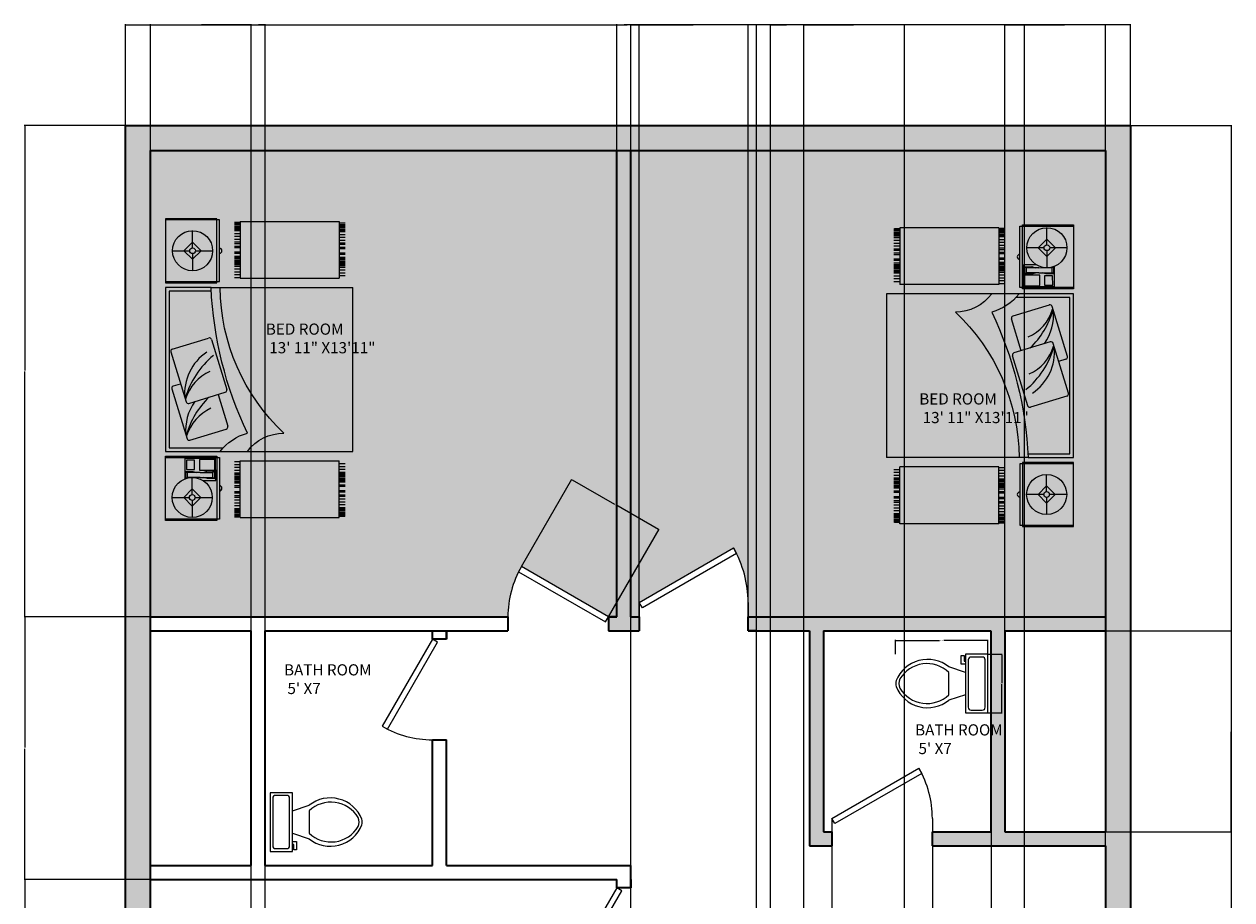
# Model space of a CAD drawing. Units: inches. Extents: x -29 to 404, y -32 to 761.
# Tile 5 of 5: x -29 to 404, y 447 to 761. Entities that reach past the tile are written whole.
import ezdxf

# ---------------------------------------------------------------- set-up
doc = ezdxf.new("R2010")
doc.units = ezdxf.units.IN
doc.header["$MEASUREMENT"] = 0
for name, color, linetype, lineweight in [('A-ANNO-DIMS', 2, 'Continuous', 18), ('A-AREA-IDEN', 7, 'Continuous', 18), ('A-FLOR-FIXT', 9, 'Continuous', 18), ('A-FURN', 8, 'Continuous', 18), ('A-WALL', 7, 'Continuous', 35), ('doors', 40, 'Continuous', 20)]:
    doc.layers.add(name, color=color, linetype=linetype, lineweight=lineweight)
doc.layers.add('A-WALL-PATT', color=251, linetype='Continuous', lineweight=13, true_color=0x636466)
doc.styles.get("Standard").update_dxf_attribs({"font": 'arial.ttf'})
doc.dimstyles.get("Standard").update_dxf_attribs({"dimtxt": 0.18, "dimasz": 0.18, "dimexe": 0.18, "dimexo": 0.0625, "dimgap": 0.09, "dimtad": 0, "dimtih": 1, "dimtoh": 1, "dimdec": 4, "dimzin": 0, "dimdsep": 46, "dimtxsty": 'Standard', "dimcen": 0.09, "dimadec": 0, "dimazin": 0, "dimtfac": 1, "dimtdec": 4, "dimtofl": 0, "dimtmove": 0, "dimatfit": 3, "dimfxl": 1, "dimtolj": 1, "dimtzin": 0, "dimarcsym": 0})

# ---------------------------------------------------------------- blocks, each defined once
blk = doc.blocks.new('3')
for p, q in [((185.866, 224.677), (185.866, 225.236)), ((185.866, 225.236), (186.566, 225.236)), ((185.88, 224.649), (185.88, 225.236)), ((186.552, 225.236), (186.552, 224.649)), ((186.566, 225.236), (186.566, 224.677)), ((186.62, 225.236), (186.62, 224.64)), ((188.409, 225.236), (186.62, 225.236)), ((187.706, 225.179), (187.161, 225.012)), ((188.409, 224.739), (188.409, 225.236)), ((188.463, 225.236), (188.463, 224.677)), ((189.162, 225.236), (188.463, 225.236)), ((188.477, 225.236), (188.477, 224.649)), ((189.148, 224.649), (189.148, 225.236)), ((189.162, 224.677), (189.162, 225.236)), ((186.022, 224.945), (186.116, 225.039)), ((186.116, 225.164), (186.116, 224.976)), ((186.116, 225.039), (186.21, 224.945)), ((187.303, 225.168), (186.758, 225.001)), ((187.334, 225.152), (187.359, 225.073)), ((187.737, 225.163), (187.858, 224.766)), ((188.812, 225.162), (188.812, 224.974)), ((186.084, 224.945), (185.896, 224.945)), ((186.116, 224.851), (186.022, 224.945)), ((186.21, 224.945), (186.116, 224.851)), ((186.116, 224.914), (186.116, 224.726)), ((186.147, 224.945), (186.335, 224.945)), ((186.54, 225.027), (186.319, 225.027)), ((186.321, 225.017), (186.401, 225.017)), ((186.333, 224.997), (186.321, 225.017)), ((186.334, 224.858), (186.333, 224.997)), ((186.333, 224.997), (186.389, 224.997)), ((186.401, 225.017), (186.389, 224.997)), ((186.39, 224.858), (186.389, 224.997)), ((186.401, 224.938), (186.389, 224.898)), ((186.401, 225.017), (186.401, 224.938)), ((186.541, 224.69), (186.54, 225.027)), ((186.742, 224.97), (186.863, 224.573)), ((187.144, 224.981), (187.266, 224.584)), ((188.781, 224.942), (188.593, 224.942)), ((188.812, 225.036), (188.718, 224.942)), ((188.718, 224.942), (188.812, 224.848)), ((188.907, 224.942), (188.812, 225.036)), ((188.812, 224.848), (188.907, 224.942)), ((188.812, 224.911), (188.812, 224.723)), ((188.844, 224.942), (189.032, 224.942)), ((186.302, 224.83), (186.303, 224.689)), ((186.322, 224.779), (186.334, 224.818)), ((186.323, 224.699), (186.322, 224.779)), ((186.331, 224.905), (186.334, 224.898)), ((186.334, 224.858), (186.334, 224.719)), ((186.39, 224.858), (186.39, 224.719)), ((186.402, 224.779), (186.39, 224.819)), ((186.402, 224.7), (186.402, 224.779)), ((186.566, 224.677), (185.866, 224.677)), ((186.552, 224.649), (185.88, 224.649)), ((186.303, 224.689), (186.541, 224.69)), ((186.334, 224.719), (186.323, 224.699)), ((186.323, 224.699), (186.402, 224.7)), ((186.334, 224.719), (186.39, 224.719)), ((186.402, 224.7), (186.39, 224.719)), ((187.242, 224.663), (186.894, 224.557)), ((187.842, 224.735), (187.297, 224.568)), ((188.409, 224.739), (188.409, 223.191)), ((188.463, 224.677), (189.162, 224.677)), ((188.477, 224.649), (189.148, 224.649)), ((186.62, 224.64), (186.62, 223.191)), ((185.897, 224.42, -0.909), (185.897, 223.338, -0.909)), ((185.897, 224.42, -0.909), (186.517, 224.42, -0.909)), ((185.904, 224.485, -0.909), (185.904, 224.42, -0.909)), ((185.92, 224.485, -0.909), (185.92, 224.42, -0.909)), ((185.92, 224.485, -0.909), (185.92, 224.42, -0.909)), ((185.935, 224.485, -0.909), (185.935, 224.42, -0.909)), ((185.951, 224.485, -0.909), (185.951, 224.42, -0.909)), ((185.966, 224.485, -0.909), (185.966, 224.42, -0.909)), ((185.982, 224.485, -0.909), (185.982, 224.42, -0.909)), ((185.997, 224.485, -0.909), (185.997, 224.42, -0.909)), ((186.028, 224.485, -0.909), (186.028, 224.42, -0.909)), ((186.059, 224.485, -0.909), (186.059, 224.42, -0.909)), ((186.09, 224.485, -0.909), (186.09, 224.42, -0.909)), ((186.09, 224.485, -0.909), (186.09, 224.42, -0.909)), ((186.121, 224.485, -0.909), (186.121, 224.42, -0.909)), ((186.137, 224.485, -0.909), (186.137, 224.42, -0.909)), ((186.168, 224.485, -0.909), (186.168, 224.42, -0.909)), ((186.183, 224.485, -0.909), (186.183, 224.42, -0.909)), ((186.23, 224.485, -0.909), (186.23, 224.42, -0.909)), ((186.245, 224.485, -0.909), (186.245, 224.42, -0.909)), ((186.276, 224.485, -0.909), (186.276, 224.42, -0.909)), ((186.292, 224.485, -0.909), (186.292, 224.42, -0.909)), ((186.307, 224.485, -0.909), (186.307, 224.42, -0.909)), ((186.323, 224.485, -0.909), (186.323, 224.42, -0.909)), ((186.338, 224.485, -0.909), (186.338, 224.42, -0.909)), ((186.354, 224.485, -0.909), (186.354, 224.42, -0.909)), ((186.369, 224.485, -0.909), (186.369, 224.42, -0.909)), ((186.385, 224.485, -0.909), (186.385, 224.42, -0.909)), ((186.416, 224.485, -0.909), (186.416, 224.42, -0.909)), ((186.447, 224.485, -0.909), (186.447, 224.42, -0.909)), ((186.478, 224.485, -0.909), (186.478, 224.42, -0.909)), ((186.509, 224.485, -0.909), (186.509, 224.42, -0.909)), ((186.517, 224.42, -0.909), (186.517, 223.338, -0.909)), ((189.131, 224.42, -0.909), (188.511, 224.42, -0.909)), ((188.511, 224.42, -0.909), (188.511, 223.338, -0.909)), ((188.52, 224.485, -0.909), (188.52, 224.42, -0.909)), ((188.551, 224.485, -0.909), (188.551, 224.42, -0.909)), ((188.582, 224.485, -0.909), (188.582, 224.42, -0.909)), ((188.613, 224.485, -0.909), (188.613, 224.42, -0.909)), ((188.644, 224.485, -0.909), (188.644, 224.42, -0.909)), ((188.66, 224.485, -0.909), (188.66, 224.42, -0.909)), ((188.675, 224.485, -0.909), (188.675, 224.42, -0.909)), ((188.691, 224.485, -0.909), (188.691, 224.42, -0.909)), ((188.706, 224.485, -0.909), (188.706, 224.42, -0.909)), ((188.722, 224.485, -0.909), (188.722, 224.42, -0.909)), ((188.737, 224.485, -0.909), (188.737, 224.42, -0.909)), ((188.753, 224.485, -0.909), (188.753, 224.42, -0.909)), ((188.784, 224.485, -0.909), (188.784, 224.42, -0.909)), ((188.799, 224.485, -0.909), (188.799, 224.42, -0.909)), ((188.846, 224.485, -0.909), (188.846, 224.42, -0.909)), ((188.861, 224.485, -0.909), (188.861, 224.42, -0.909)), ((188.892, 224.485, -0.909), (188.892, 224.42, -0.909)), ((188.908, 224.485, -0.909), (188.908, 224.42, -0.909)), ((188.939, 224.485, -0.909), (188.939, 224.42, -0.909)), ((188.939, 224.485, -0.909), (188.939, 224.42, -0.909)), ((188.97, 224.485, -0.909), (188.97, 224.42, -0.909)), ((189.001, 224.485, -0.909), (189.001, 224.42, -0.909)), ((189.032, 224.485, -0.909), (189.032, 224.42, -0.909)), ((189.047, 224.485, -0.909), (189.047, 224.42, -0.909)), ((189.063, 224.485, -0.909), (189.063, 224.42, -0.909)), ((189.078, 224.485, -0.909), (189.078, 224.42, -0.909)), ((189.094, 224.485, -0.909), (189.094, 224.42, -0.909)), ((189.109, 224.485, -0.909), (189.109, 224.42, -0.909)), ((189.109, 224.485, -0.909), (189.109, 224.42, -0.909)), ((189.125, 224.485, -0.909), (189.125, 224.42, -0.909)), ((189.131, 224.42, -0.909), (189.131, 223.338, -0.909)), ((185.897, 223.338, -0.909), (186.517, 223.338, -0.909)), ((185.911, 223.338, -0.909), (185.911, 223.279, -0.909)), ((185.911, 223.338, -0.909), (185.911, 223.279, -0.909)), ((185.911, 223.338, -0.909), (185.911, 223.279, -0.909)), ((185.914, 223.338, -0.909), (185.914, 223.273, -0.909)), ((185.929, 223.338, -0.909), (185.929, 223.273, -0.909)), ((185.929, 223.338, -0.909), (185.929, 223.273, -0.909)), ((185.945, 223.338, -0.909), (185.945, 223.273, -0.909)), ((185.96, 223.338, -0.909), (185.96, 223.273, -0.909)), ((185.976, 223.338, -0.909), (185.976, 223.273, -0.909)), ((185.991, 223.338, -0.909), (185.991, 223.273, -0.909)), ((186.007, 223.338, -0.909), (186.007, 223.273, -0.909)), ((186.038, 223.338, -0.909), (186.038, 223.273, -0.909)), ((186.069, 223.338, -0.909), (186.069, 223.273, -0.909)), ((186.1, 223.338, -0.909), (186.1, 223.273, -0.909)), ((186.1, 223.338, -0.909), (186.1, 223.273, -0.909)), ((186.131, 223.338, -0.909), (186.131, 223.273, -0.909)), ((186.146, 223.338, -0.909), (186.146, 223.273, -0.909)), ((186.177, 223.338, -0.909), (186.177, 223.273, -0.909)), ((186.193, 223.338, -0.909), (186.193, 223.273, -0.909)), ((186.239, 223.338, -0.909), (186.239, 223.273, -0.909)), ((186.255, 223.338, -0.909), (186.255, 223.273, -0.909)), ((186.286, 223.338, -0.909), (186.286, 223.273, -0.909)), ((186.301, 223.338, -0.909), (186.301, 223.273, -0.909)), ((186.317, 223.338, -0.909), (186.317, 223.273, -0.909)), ((186.332, 223.338, -0.909), (186.332, 223.273, -0.909)), ((186.348, 223.338, -0.909), (186.348, 223.273, -0.909)), ((186.363, 223.338, -0.909), (186.363, 223.273, -0.909)), ((186.379, 223.338, -0.909), (186.379, 223.273, -0.909)), ((186.394, 223.338, -0.909), (186.394, 223.273, -0.909)), ((186.425, 223.338, -0.909), (186.425, 223.273, -0.909)), ((186.456, 223.338, -0.909), (186.456, 223.273, -0.909)), ((186.487, 223.338, -0.909), (186.487, 223.273, -0.909)), ((189.131, 223.338, -0.909), (188.511, 223.338, -0.909)), ((188.541, 223.338, -0.909), (188.541, 223.273, -0.909)), ((188.572, 223.338, -0.909), (188.572, 223.273, -0.909)), ((188.603, 223.338, -0.909), (188.603, 223.273, -0.909)), ((188.634, 223.338, -0.909), (188.634, 223.273, -0.909)), ((188.65, 223.338, -0.909), (188.65, 223.273, -0.909)), ((188.665, 223.338, -0.909), (188.665, 223.273, -0.909)), ((188.681, 223.338, -0.909), (188.681, 223.273, -0.909)), ((188.696, 223.338, -0.909), (188.696, 223.273, -0.909)), ((188.712, 223.338, -0.909), (188.712, 223.273, -0.909)), ((188.727, 223.338, -0.909), (188.727, 223.273, -0.909)), ((188.743, 223.338, -0.909), (188.743, 223.273, -0.909)), ((188.774, 223.338, -0.909), (188.774, 223.273, -0.909)), ((188.789, 223.338, -0.909), (188.789, 223.273, -0.909)), ((188.836, 223.338, -0.909), (188.836, 223.273, -0.909)), ((188.851, 223.338, -0.909), (188.851, 223.273, -0.909)), ((188.882, 223.338, -0.909), (188.882, 223.273, -0.909)), ((188.898, 223.338, -0.909), (188.898, 223.273, -0.909)), ((188.929, 223.338, -0.909), (188.929, 223.273, -0.909)), ((188.929, 223.338, -0.909), (188.929, 223.273, -0.909)), ((188.96, 223.338, -0.909), (188.96, 223.273, -0.909)), ((188.991, 223.338, -0.909), (188.991, 223.273, -0.909)), ((189.022, 223.338, -0.909), (189.022, 223.273, -0.909)), ((189.037, 223.338, -0.909), (189.037, 223.273, -0.909)), ((189.053, 223.338, -0.909), (189.053, 223.273, -0.909)), ((189.068, 223.338, -0.909), (189.068, 223.273, -0.909)), ((189.084, 223.338, -0.909), (189.084, 223.273, -0.909)), ((189.099, 223.338, -0.909), (189.099, 223.273, -0.909)), ((189.099, 223.338, -0.909), (189.099, 223.273, -0.909)), ((189.115, 223.338, -0.909), (189.115, 223.273, -0.909)), ((189.117, 223.338, -0.909), (189.117, 223.279, -0.909)), ((189.117, 223.338, -0.909), (189.117, 223.279, -0.909)), ((189.117, 223.338, -0.909), (189.117, 223.279, -0.909)), ((186.62, 223.191), (188.409, 223.191))]:
    blk.add_line(p, q)
blk.add_lwpolyline([(188.369, 224.737), (188.369, 225.197), (186.66, 225.197), (186.66, 224.606)])
for points in [[(186.422, 225.007), (186.422, 224.92), (186.525, 224.92), (186.525, 225.008)], [(186.415, 224.866), (186.416, 224.7), (186.531, 224.7), (186.53, 224.867)]]:
    blk.add_lwpolyline(points, close=True)
for points in [[(186.62, 224.64, -0.162278), (186.819, 224.342, -0.100664), (188.409, 224.739, -0.100664)], [(186.62, 224.342, -0.236068), (186.819, 223.944, -0.205258), (188.409, 224.64, -0.205258)]]:
    blk.add_lwpolyline(points, format="xyb")
for centre, radius in [((186.116, 224.945), 0.219), ((188.812, 224.942), 0.219), ((186.116, 224.945), 0.0313), ((188.812, 224.942), 0.0313)]:
    blk.add_circle(centre, radius)
for centre, radius, start, end in [((187.713, 225.156), 0.0248, 17.0142, 107.0142), ((187.311, 225.145), 0.0248, 17.0142, 107.0142), ((186.765, 224.978), 0.0248, 107.0142, 197.0142), ((186.647, 224.541), 0.487, 24.2209, 73.0691), ((186.848, 224.471), 0.547, 54.6851, 95.1605), ((186.536, 224.105), 0.943, 44.2727, 73.7189), ((187.168, 224.989), 0.0248, 107.0142, 197.0142), ((187.05, 224.552), 0.487, 24.2209, 73.0691), ((187.25, 224.482), 0.547, 33.7801, 95.1605), ((186.938, 224.116), 0.943, 39.4023, 73.7189), ((186.216, 224.649), 0.028, 180, 0), ((187.835, 224.758), 0.0248, 287.0142, 17.0142), ((188.812, 224.649), 0.028, 180, 0), ((186.887, 224.581), 0.0248, 197.0142, 287.0142), ((187.289, 224.592), 0.0248, 197.0142, 287.0142)]:
    blk.add_arc(centre, radius, start, end)
blk = doc.blocks.new('Toilet - top')
for p, q in [((9.5, -6), (9.5, -2)), ((-10, -8.5), (-8, -8.5)), ((-10, -9.5), (-10, -8.5)), ((-8, -8.5), (-8, -8)), ((-7, -8), (-7, -9.5)), ((-4, -8), (-6, -14)), ((4, -8), (6, -14)), ((-7, -9.5), (-10, -9.5)), ((4, -14), (-4, -14))]:
    blk.add_line(p, q)
blk.add_lwpolyline([(10.5, -8), (10.5, 0), (-10.5, 0), (-10.5, -8)], close=True)
for points in [[(-9.5, -2), (-9.5, -6)], [(8.5, -1), (-8.5, -1)], [(-8.5, -7), (8.5, -7)]]:
    blk.add_lwpolyline(points)
for centre, radius, start, end in [((-8.62, -1.88), 0.884, 81.8699, 188.1301), ((8.62, -1.88), 0.884, 351.8699, 98.1301), ((-8.62, -6.12), 0.884, 171.8699, 278.1301), ((8.62, -6.12), 0.884, 261.8699, 8.1301), ((3.52, -21.58), 12.17, 141.4691, 247.9714), ((4.2, -21.82), 11.33, 136.3677, 238.9468), ((-3.52, -21.58), 12.17, 292.0284, 38.5307), ((-4.2, -21.82), 11.33, 301.053, 43.6321), ((0, -27.88), 4, 245.7318, 294.2682), ((0, -29), 4, 254.8605, 285.1395)]:
    blk.add_arc(centre, radius, start, end)
blk = doc.blocks.new('*U7')
for p, q in [((0, 0), (0, 100)), ((750, 0), (750, 100))]:
    blk.add_line(p, q)
blk.add_lwpolyline([(0, 0), (649.5, -375), (671.4, -337.1), (21.9, 37.9)], close=True)
blk.add_arc((0, 0), 750, 330, 0)
blk = doc.blocks.new('*U6')
for p, q in [((0, 0), (0, -100)), ((750, 0), (750, -100))]:
    blk.add_line(p, q)
blk.add_lwpolyline([(0, 0), (649.5, 375), (671.4, 337.1), (21.9, -37.9)], close=True)
blk.add_arc((0, 0), 750, 0, 30)
blk = doc.blocks.new('*D15')
at = {"layer": 'A-ANNO-DIMS', "color": 0, "lineweight": -2, "transparency": 16777216}
for p, q in [((283.5, 535.13), (283.5, 540.2)), ((283.68, 540.02), (299.25, 540.02)), ((316.37, 540.02), (300.8, 540.02)), ((316.55, 535.13), (316.55, 540.2))]:
    blk.add_line(p, q, dxfattribs=at)
at = {"layer": 'A-ANNO-DIMS', "color": 0, "transparency": 16777216}
for points in [[(283.68, 540.05), (283.68, 539.99), (283.5, 540.02)], [(316.37, 540.05), (316.37, 539.99), (316.55, 540.02)]]:
    blk.add_solid(points, dxfattribs=at)
at = {"layer": 'Defpoints', "color": 0, "transparency": 16777216}
for p in [(316.55, 540.02), (283.5, 535.07), (316.55, 535.07)]:
    blk.add_point(p, dxfattribs=at)
at = {"layer": 'A-ANNO-DIMS', "color": 0, "transparency": 16777216, "insert": (300.03, 540.02), "char_height": 0.18, "attachment_point": 5}
blk.add_mtext('\\A1;WC 33 TYP.', dxfattribs=at)
blk = doc.blocks.new('*D16')
at = {"layer": 'A-ANNO-DIMS', "color": 0, "lineweight": -2, "transparency": 16777216}
for p, q in [((316.61, 535.07), (321.69, 535.07)), ((321.51, 534.89), (321.51, 524.75)), ((321.51, 514.25), (321.51, 524.39)), ((316.61, 514.07), (321.69, 514.07))]:
    blk.add_line(p, q, dxfattribs=at)
at = {"layer": 'A-ANNO-DIMS', "color": 0, "transparency": 16777216}
for points in [[(321.48, 534.89), (321.54, 534.89), (321.51, 535.07)], [(321.48, 514.25), (321.54, 514.25), (321.51, 514.07)]]:
    blk.add_solid(points, dxfattribs=at)
at = {"layer": 'Defpoints', "color": 0, "transparency": 16777216}
for p in [(316.55, 535.07), (316.55, 514.07), (321.51, 514.07)]:
    blk.add_point(p, dxfattribs=at)
at = {"layer": 'A-ANNO-DIMS', "color": 0, "transparency": 16777216, "insert": (321.51, 524.57), "char_height": 0.18, "attachment_point": 5}
blk.add_mtext('\\A1;21 TYP.', dxfattribs=at)
blk = doc.blocks.new('*D31')
at = {"layer": 'A-ANNO-DIMS', "color": 0, "lineweight": -2, "transparency": 16777216}
for p, q in [((7.68, 724.5), (7.68, 760.66)), ((7.86, 760.48), (187.39, 760.48)), ((367.5, 760.48), (187.97, 760.48)), ((367.68, 724.5), (367.68, 760.66))]:
    blk.add_line(p, q, dxfattribs=at)
at = {"layer": 'A-ANNO-DIMS', "color": 0, "transparency": 16777216}
for points in [[(7.86, 760.51), (7.86, 760.45), (7.68, 760.48)], [(367.5, 760.51), (367.5, 760.45), (367.68, 760.48)]]:
    blk.add_solid(points, dxfattribs=at)
at = {"layer": 'Defpoints', "color": 0, "transparency": 16777216}
for p in [(367.68, 760.48), (7.68, 724.43), (367.68, 724.43)]:
    blk.add_point(p, dxfattribs=at)
at = {"layer": 'A-ANNO-DIMS', "color": 0, "transparency": 16777216, "insert": (187.68, 760.48), "char_height": 0.18, "attachment_point": 5}
blk.add_mtext('\\A1;360', dxfattribs=at)
blk = doc.blocks.new('*D32')
at = {"layer": 'A-ANNO-DIMS', "color": 0, "lineweight": -2, "transparency": 16777216}
for p, q in [((367.74, 724.43), (403.91, 724.43)), ((403.73, 724.25), (403.73, 364.62)), ((403.73, 4.61), (403.73, 364.25)), ((367.74, 4.43), (403.91, 4.43))]:
    blk.add_line(p, q, dxfattribs=at)
at = {"layer": 'A-ANNO-DIMS', "color": 0, "transparency": 16777216}
for points in [[(403.7, 724.25), (403.76, 724.25), (403.73, 724.43)], [(403.7, 4.61), (403.76, 4.61), (403.73, 4.43)]]:
    blk.add_solid(points, dxfattribs=at)
at = {"layer": 'Defpoints', "color": 0, "transparency": 16777216}
for p in [(367.68, 724.43), (403.73, 724.43), (367.68, 4.43)]:
    blk.add_point(p, dxfattribs=at)
at = {"layer": 'A-ANNO-DIMS', "color": 0, "transparency": 16777216, "insert": (403.73, 364.43), "char_height": 0.18, "attachment_point": 5}
blk.add_mtext('\\A1;720', dxfattribs=at)
blk = doc.blocks.new('*D35')
at = {"layer": 'A-ANNO-DIMS', "color": 0, "lineweight": -2, "transparency": 16777216}
for p, q in [((16.62, 454.43), (-28.55, 454.43)), ((-28.37, 454.25), (-28.37, 371.12)), ((-28.37, 287.61), (-28.37, 370.75)), ((16.62, 287.43), (-28.55, 287.43))]:
    blk.add_line(p, q, dxfattribs=at)
at = {"layer": 'A-ANNO-DIMS', "color": 0, "transparency": 16777216}
for points in [[(-28.4, 454.25), (-28.34, 454.25), (-28.37, 454.43)], [(-28.4, 287.61), (-28.34, 287.61), (-28.37, 287.43)]]:
    blk.add_solid(points, dxfattribs=at)
at = {"layer": 'Defpoints', "color": 0, "transparency": 16777216}
for p in [(-28.37, 454.43), (16.68, 454.43), (16.68, 287.43)]:
    blk.add_point(p, dxfattribs=at)
at = {"layer": 'A-ANNO-DIMS', "color": 0, "transparency": 16777216, "insert": (-28.37, 370.93), "char_height": 0.18, "attachment_point": 5}
blk.add_mtext('\\A1;167', dxfattribs=at)
blk = doc.blocks.new('*D36')
at = {"layer": 'A-ANNO-DIMS', "color": 0, "lineweight": -2, "transparency": 16777216}
for p, q in [((16.62, 548.43), (-28.55, 548.43)), ((-28.37, 548.25), (-28.37, 501.62)), ((-28.37, 454.61), (-28.37, 501.25)), ((16.62, 454.43), (-28.55, 454.43))]:
    blk.add_line(p, q, dxfattribs=at)
at = {"layer": 'A-ANNO-DIMS', "color": 0, "transparency": 16777216}
for points in [[(-28.4, 548.25), (-28.34, 548.25), (-28.37, 548.43)], [(-28.4, 454.61), (-28.34, 454.61), (-28.37, 454.43)]]:
    blk.add_solid(points, dxfattribs=at)
at = {"layer": 'Defpoints', "color": 0, "transparency": 16777216}
for p in [(-28.37, 548.43), (16.68, 548.43), (16.68, 454.43)]:
    blk.add_point(p, dxfattribs=at)
at = {"layer": 'A-ANNO-DIMS', "color": 0, "transparency": 16777216, "insert": (-28.37, 501.43), "char_height": 0.18, "attachment_point": 5}
blk.add_mtext('\\A1;94', dxfattribs=at)
blk = doc.blocks.new('*D37')
at = {"layer": 'A-ANNO-DIMS', "color": 0, "lineweight": -2, "transparency": 16777216}
for p, q in [((7.62, 724.43), (-28.55, 724.43)), ((-28.37, 724.25), (-28.37, 636.62)), ((-28.37, 548.61), (-28.37, 636.25)), ((16.62, 548.43), (-28.55, 548.43))]:
    blk.add_line(p, q, dxfattribs=at)
at = {"layer": 'A-ANNO-DIMS', "color": 0, "transparency": 16777216}
for points in [[(-28.4, 724.25), (-28.34, 724.25), (-28.37, 724.43)], [(-28.4, 548.61), (-28.34, 548.61), (-28.37, 548.43)]]:
    blk.add_solid(points, dxfattribs=at)
at = {"layer": 'Defpoints', "color": 0, "transparency": 16777216}
for p in [(-28.37, 724.43), (7.68, 724.43), (16.68, 548.43)]:
    blk.add_point(p, dxfattribs=at)
at = {"layer": 'A-ANNO-DIMS', "color": 0, "transparency": 16777216, "insert": (-28.37, 636.43), "char_height": 0.18, "attachment_point": 5}
blk.add_mtext('\\A1;176', dxfattribs=at)
blk = doc.blocks.new('*D41')
at = {"layer": 'A-ANNO-DIMS', "color": 0, "lineweight": -2, "transparency": 16777216}
for p, q in [((250.68, 193.5), (250.68, 760.66)), ((250.86, 760.48), (268.46, 760.48)), ((286.5, 760.48), (268.9, 760.48)), ((286.68, 193.5), (286.68, 760.66))]:
    blk.add_line(p, q, dxfattribs=at)
at = {"layer": 'A-ANNO-DIMS', "color": 0, "transparency": 16777216}
for points in [[(250.86, 760.51), (250.86, 760.45), (250.68, 760.48)], [(286.5, 760.51), (286.5, 760.45), (286.68, 760.48)]]:
    blk.add_solid(points, dxfattribs=at)
at = {"layer": 'Defpoints', "color": 0, "transparency": 16777216}
for p in [(286.68, 760.48), (250.68, 193.43), (286.68, 193.43)]:
    blk.add_point(p, dxfattribs=at)
at = {"layer": 'A-ANNO-DIMS', "color": 0, "transparency": 16777216, "insert": (268.68, 760.48), "char_height": 0.18, "attachment_point": 5}
blk.add_mtext('\\A1;36', dxfattribs=at)
blk = doc.blocks.new('*D42')
at = {"layer": 'A-ANNO-DIMS', "color": 0, "lineweight": -2, "transparency": 16777216}
for p, q in [((238.68, 193.5), (238.68, 760.66)), ((238.86, 760.48), (244.47, 760.48)), ((250.5, 760.48), (244.89, 760.48)), ((250.68, 193.5), (250.68, 760.66))]:
    blk.add_line(p, q, dxfattribs=at)
at = {"layer": 'A-ANNO-DIMS', "color": 0, "transparency": 16777216}
for points in [[(238.86, 760.51), (238.86, 760.45), (238.68, 760.48)], [(250.5, 760.51), (250.5, 760.45), (250.68, 760.48)]]:
    blk.add_solid(points, dxfattribs=at)
at = {"layer": 'Defpoints', "color": 0, "transparency": 16777216}
for p in [(250.68, 760.48), (238.68, 193.43), (250.68, 193.43)]:
    blk.add_point(p, dxfattribs=at)
at = {"layer": 'A-ANNO-DIMS', "color": 0, "transparency": 16777216, "insert": (244.68, 760.48), "char_height": 0.18, "attachment_point": 5}
blk.add_mtext('\\A1;12', dxfattribs=at)
blk = doc.blocks.new('*D44')
at = {"layer": 'A-ANNO-DIMS', "color": 0, "lineweight": -2, "transparency": 16777216}
for p, q in [((188.68, 92.5), (188.68, 760.66)), ((188.86, 760.48), (210.95, 760.48)), ((233.5, 760.48), (211.4, 760.48)), ((233.68, 92.5), (233.68, 760.66))]:
    blk.add_line(p, q, dxfattribs=at)
at = {"layer": 'A-ANNO-DIMS', "color": 0, "transparency": 16777216}
for points in [[(188.86, 760.51), (188.86, 760.45), (188.68, 760.48)], [(233.5, 760.51), (233.5, 760.45), (233.68, 760.48)]]:
    blk.add_solid(points, dxfattribs=at)
at = {"layer": 'Defpoints', "color": 0, "transparency": 16777216}
for p in [(233.68, 760.48), (188.68, 92.43), (233.68, 92.43)]:
    blk.add_point(p, dxfattribs=at)
at = {"layer": 'A-ANNO-DIMS', "color": 0, "transparency": 16777216, "insert": (211.18, 760.48), "char_height": 0.18, "attachment_point": 5}
blk.add_mtext('\\A1;45', dxfattribs=at)
blk = doc.blocks.new('*D45')
at = {"layer": 'A-ANNO-DIMS', "color": 0, "lineweight": -2, "transparency": 16777216}
for p, q in [((329.68, 126.5), (329.68, 760.66)), ((329.86, 760.48), (343.96, 760.48)), ((358.5, 760.48), (344.4, 760.48)), ((358.68, 97.5), (358.68, 760.66))]:
    blk.add_line(p, q, dxfattribs=at)
at = {"layer": 'A-ANNO-DIMS', "color": 0, "transparency": 16777216}
for points in [[(329.86, 760.51), (329.86, 760.45), (329.68, 760.48)], [(358.5, 760.51), (358.5, 760.45), (358.68, 760.48)]]:
    blk.add_solid(points, dxfattribs=at)
at = {"layer": 'Defpoints', "color": 0, "transparency": 16777216}
for p in [(358.68, 760.48), (329.68, 126.43), (358.68, 97.43)]:
    blk.add_point(p, dxfattribs=at)
at = {"layer": 'A-ANNO-DIMS', "color": 0, "transparency": 16777216, "insert": (344.18, 760.48), "char_height": 0.18, "attachment_point": 5}
blk.add_mtext('\\A1;29', dxfattribs=at)
blk = doc.blocks.new('*D48')
at = {"layer": 'A-ANNO-DIMS', "color": 0, "lineweight": -2, "transparency": 16777216}
for p, q in [((183.68, 715.5), (183.68, 760.66)), ((183.86, 760.48), (186.03, 760.48)), ((188.5, 760.48), (186.33, 760.48)), ((188.68, 715.5), (188.68, 760.66))]:
    blk.add_line(p, q, dxfattribs=at)
at = {"layer": 'A-ANNO-DIMS', "color": 0, "transparency": 16777216}
for points in [[(183.86, 760.51), (183.86, 760.45), (183.68, 760.48)], [(188.5, 760.51), (188.5, 760.45), (188.68, 760.48)]]:
    blk.add_solid(points, dxfattribs=at)
at = {"layer": 'Defpoints', "color": 0, "transparency": 16777216}
for p in [(188.68, 760.48), (183.68, 715.43), (188.68, 715.43)]:
    blk.add_point(p, dxfattribs=at)
at = {"layer": 'A-ANNO-DIMS', "color": 0, "transparency": 16777216, "insert": (186.18, 760.48), "char_height": 0.18, "attachment_point": 5}
blk.add_mtext('\\A1;5', dxfattribs=at)
blk = doc.blocks.new('*D50')
at = {"layer": 'A-ANNO-DIMS', "color": 0, "lineweight": -2, "transparency": 16777216}
for p, q in [((260.68, 466.37), (260.68, -31.8)), ((296.68, 466.37), (296.68, -31.8)), ((260.86, -31.62), (278.46, -31.62)), ((296.5, -31.62), (278.9, -31.62))]:
    blk.add_line(p, q, dxfattribs=at)
at = {"layer": 'A-ANNO-DIMS', "color": 0, "transparency": 16777216}
for points in [[(260.86, -31.59), (260.86, -31.65), (260.68, -31.62)], [(296.5, -31.59), (296.5, -31.65), (296.68, -31.62)]]:
    blk.add_solid(points, dxfattribs=at)
at = {"layer": 'Defpoints', "color": 0, "transparency": 16777216}
for p in [(260.68, 466.43), (296.68, 466.43), (296.68, -31.62)]:
    blk.add_point(p, dxfattribs=at)
at = {"layer": 'A-ANNO-DIMS', "color": 0, "transparency": 16777216, "insert": (278.68, -31.62), "char_height": 0.18, "attachment_point": 5}
blk.add_mtext('\\A1;36', dxfattribs=at)
blk = doc.blocks.new('*D51')
at = {"layer": 'A-ANNO-DIMS', "color": 0, "lineweight": -2, "transparency": 16777216}
for p, q in [((296.68, 471.37), (296.68, -31.8)), ((317.68, 471.37), (317.68, -31.8)), ((296.86, -31.62), (306.97, -31.62)), ((317.5, -31.62), (307.38, -31.62))]:
    blk.add_line(p, q, dxfattribs=at)
at = {"layer": 'A-ANNO-DIMS', "color": 0, "transparency": 16777216}
for points in [[(296.86, -31.59), (296.86, -31.65), (296.68, -31.62)], [(317.5, -31.59), (317.5, -31.65), (317.68, -31.62)]]:
    blk.add_solid(points, dxfattribs=at)
at = {"layer": 'Defpoints', "color": 0, "transparency": 16777216}
for p in [(296.68, 471.43), (317.68, 471.43), (317.68, -31.62)]:
    blk.add_point(p, dxfattribs=at)
at = {"layer": 'A-ANNO-DIMS', "color": 0, "transparency": 16777216, "insert": (307.18, -31.62), "char_height": 0.18, "attachment_point": 5}
blk.add_mtext('\\A1;21', dxfattribs=at)
blk = doc.blocks.new('*D52')
at = {"layer": 'A-ANNO-DIMS', "color": 0, "lineweight": -2, "transparency": 16777216}
for p, q in [((358.74, 543.43), (403.91, 543.43)), ((403.73, 543.25), (403.73, 507.61)), ((403.73, 471.61), (403.73, 507.25)), ((358.74, 471.43), (403.91, 471.43))]:
    blk.add_line(p, q, dxfattribs=at)
at = {"layer": 'A-ANNO-DIMS', "color": 0, "transparency": 16777216}
for points in [[(403.7, 543.25), (403.76, 543.25), (403.73, 543.43)], [(403.7, 471.61), (403.76, 471.61), (403.73, 471.43)]]:
    blk.add_solid(points, dxfattribs=at)
at = {"layer": 'Defpoints', "color": 0, "transparency": 16777216}
for p in [(358.68, 543.43), (403.73, 543.43), (358.68, 471.43)]:
    blk.add_point(p, dxfattribs=at)
at = {"layer": 'A-ANNO-DIMS', "color": 0, "transparency": 16777216, "insert": (403.73, 507.43), "char_height": 0.18, "attachment_point": 5}
blk.add_mtext('\\A1;72', dxfattribs=at)
blk = doc.blocks.new('*D53')
at = {"layer": 'A-ANNO-DIMS', "color": 0, "lineweight": -2, "transparency": 16777216}
for p, q in [((322.68, 543.5), (322.68, 760.66)), ((322.86, 760.48), (340.46, 760.48)), ((358.5, 760.48), (340.9, 760.48)), ((358.68, 543.5), (358.68, 760.66))]:
    blk.add_line(p, q, dxfattribs=at)
at = {"layer": 'A-ANNO-DIMS', "color": 0, "transparency": 16777216}
for points in [[(322.86, 760.51), (322.86, 760.45), (322.68, 760.48)], [(358.5, 760.51), (358.5, 760.45), (358.68, 760.48)]]:
    blk.add_solid(points, dxfattribs=at)
at = {"layer": 'Defpoints', "color": 0, "transparency": 16777216}
for p in [(358.68, 760.48), (322.68, 543.43), (358.68, 543.43)]:
    blk.add_point(p, dxfattribs=at)
at = {"layer": 'A-ANNO-DIMS', "color": 0, "transparency": 16777216, "insert": (340.68, 760.48), "char_height": 0.18, "attachment_point": 5}
blk.add_mtext('\\A1;36', dxfattribs=at)
blk = doc.blocks.new('*D56')
at = {"layer": 'A-ANNO-DIMS', "color": 0, "lineweight": -2, "transparency": 16777216}
for p, q in [((149.53, 566.49), (167.62, 597.81)), ((167.68, 597.56), (182.9, 588.78)), ((198.55, 579.74), (183.33, 588.53)), ((180.71, 548.49), (198.79, 579.81))]:
    blk.add_line(p, q, dxfattribs=at)
at = {"layer": 'A-ANNO-DIMS', "color": 0, "transparency": 16777216}
for points in [[(167.7, 597.59), (167.67, 597.54), (167.53, 597.65)], [(198.56, 579.77), (198.53, 579.72), (198.7, 579.65)]]:
    blk.add_solid(points, dxfattribs=at)
at = {"layer": 'Defpoints', "color": 0, "transparency": 16777216}
for p in [(198.7, 579.65), (149.5, 566.43), (180.68, 548.43)]:
    blk.add_point(p, dxfattribs=at)
at = {"layer": 'A-ANNO-DIMS', "color": 0, "transparency": 16777216, "insert": (183.11, 588.65), "char_height": 0.18, "attachment_point": 5}
blk.add_mtext('\\A1;36', dxfattribs=at)
blk = doc.blocks.new('*D57')
at = {"layer": 'A-ANNO-DIMS', "color": 0, "lineweight": -2, "transparency": 16777216}
for p, q in [((191.68, 543.5), (191.68, 760.66)), ((191.86, 760.48), (210.96, 760.48)), ((230.5, 760.48), (211.4, 760.48)), ((230.68, 543.5), (230.68, 760.66))]:
    blk.add_line(p, q, dxfattribs=at)
at = {"layer": 'A-ANNO-DIMS', "color": 0, "transparency": 16777216}
for points in [[(191.86, 760.51), (191.86, 760.45), (191.68, 760.48)], [(230.5, 760.51), (230.5, 760.45), (230.68, 760.48)]]:
    blk.add_solid(points, dxfattribs=at)
at = {"layer": 'Defpoints', "color": 0, "transparency": 16777216}
for p in [(230.68, 760.48), (191.68, 543.43), (230.68, 543.43)]:
    blk.add_point(p, dxfattribs=at)
at = {"layer": 'A-ANNO-DIMS', "color": 0, "transparency": 16777216, "insert": (211.18, 760.48), "char_height": 0.18, "attachment_point": 5}
blk.add_mtext('\\A1;39', dxfattribs=at)
blk = doc.blocks.new('*D59')
at = {"layer": 'A-ANNO-DIMS', "color": 0, "lineweight": -2, "transparency": 16777216}
for p, q in [((16.68, 198.5), (16.68, 760.66)), ((16.86, 760.48), (34.46, 760.48)), ((52.5, 760.48), (34.9, 760.48)), ((52.68, 198.5), (52.68, 760.66))]:
    blk.add_line(p, q, dxfattribs=at)
at = {"layer": 'A-ANNO-DIMS', "color": 0, "transparency": 16777216}
for points in [[(16.86, 760.51), (16.86, 760.45), (16.68, 760.48)], [(52.5, 760.51), (52.5, 760.45), (52.68, 760.48)]]:
    blk.add_solid(points, dxfattribs=at)
at = {"layer": 'Defpoints', "color": 0, "transparency": 16777216}
for p in [(52.68, 760.48), (16.68, 198.43), (52.68, 198.43)]:
    blk.add_point(p, dxfattribs=at)
at = {"layer": 'A-ANNO-DIMS', "color": 0, "transparency": 16777216, "insert": (34.68, 760.48), "char_height": 0.18, "attachment_point": 5}
blk.add_mtext('\\A1;36', dxfattribs=at)
blk = doc.blocks.new('*D60')
at = {"layer": 'A-ANNO-DIMS', "color": 0, "lineweight": -2, "transparency": 16777216}
for p, q in [((52.68, 198.5), (52.68, 760.66)), ((52.86, 760.48), (55.03, 760.48)), ((57.5, 760.48), (55.33, 760.48)), ((57.68, 198.5), (57.68, 760.66))]:
    blk.add_line(p, q, dxfattribs=at)
at = {"layer": 'A-ANNO-DIMS', "color": 0, "transparency": 16777216}
for points in [[(52.86, 760.51), (52.86, 760.45), (52.68, 760.48)], [(57.5, 760.51), (57.5, 760.45), (57.68, 760.48)]]:
    blk.add_solid(points, dxfattribs=at)
at = {"layer": 'Defpoints', "color": 0, "transparency": 16777216}
for p in [(57.68, 760.48), (52.68, 198.43), (57.68, 198.43)]:
    blk.add_point(p, dxfattribs=at)
at = {"layer": 'A-ANNO-DIMS', "color": 0, "transparency": 16777216, "insert": (55.18, 760.48), "char_height": 0.18, "attachment_point": 5}
blk.add_mtext('\\A1;5', dxfattribs=at)

msp = doc.modelspace()

# ---------------------------------------------------------------- hatches: boundary and pattern name
at = {"layer": 'A-WALL-PATT'}
h = msp.add_hatch(color=256, dxfattribs=at)
h.dxf.hatch_style = 1
h.paths.add_polyline_path([(188.678, 415.434), (183.678, 415.434), (183.678, 287.434), (180.678, 287.434), (180.678, 282.434), (183.678, 282.434), (183.678, 198.434), (57.678, 198.434), (57.678, 282.434), (144.678, 282.434), (144.678, 287.434), (16.678, 287.434), (16.678, 548.434), (144.678, 548.434, -0.1168354), (148.504, 564.585), (148.451, 564.616), (149.501, 566.434), (180.678, 548.434), (180.678, 543.434), (183.678, 543.434), (191.678, 543.434), (191.678, 548.434), (191.678, 553.634), (225.453, 573.134), (226.591, 571.164), (226.533, 571.131, -0.1168354), (230.678, 553.634), (230.678, 548.434), (358.678, 548.434), (358.678, 471.434), (322.678, 471.434), (322.678, 543.434), (358.678, 543.434), (358.678, 548.434), (230.678, 548.434), (230.678, 543.434), (233.678, 543.434), (252.678, 543.434), (252.678, 466.434), (260.678, 466.434), (260.678, 471.434), (257.678, 471.434), (257.678, 543.434), (317.678, 543.434), (317.678, 471.434), (296.678, 471.434), (296.678, 466.434), (358.678, 466.434), (358.678, 198.434), (286.678, 198.434), (286.678, 193.434), (358.678, 193.434), (358.678, 97.434), (238.678, 97.434), (238.678, 193.434), (250.678, 193.434), (250.678, 198.434), (233.678, 198.434), (233.678, 92.434), (358.678, 92.434), (358.678, 13.434), (296.678, 13.434), (296.678, 4.434), (367.678, 4.434), (367.678, 724.434), (7.678, 724.434), (7.678, 4.434), (188.678, 4.434), (188.678, 13.434), (188.678, 154.434), (183.678, 154.434), (183.678, 13.434), (49.651, 13.434), (48.286, 12.069), (46.92, 13.434), (16.678, 13.434), (16.678, 193.434), (183.678, 193.434), (183.678, 190.434), (188.678, 190.434)])
h.paths.add_polyline_path([(52.678, 282.434), (52.678, 198.434), (16.678, 198.434), (16.678, 282.434)], flags=16)

# ---------------------------------------------------------------- linework, layer by layer
at = {"layer": 'A-WALL'}
for p, q in [((16.678, 715.434), (358.678, 715.434)), ((16.678, 287.434), (16.678, 715.434)), ((183.678, 548.434), (183.678, 715.434)), ((188.678, 548.434), (188.678, 715.434)), ((358.678, 715.434), (358.678, 471.434)), ((16.678, 548.434), (144.678, 548.434)), ((144.678, 548.434), (144.678, 543.434)), ((180.678, 548.434), (183.678, 548.434)), ((183.678, 548.434), (180.678, 548.434)), ((180.678, 548.434), (180.678, 543.434)), ((188.678, 548.434), (191.678, 548.434)), ((188.678, 548.434), (191.678, 548.434)), ((191.678, 548.434), (191.678, 543.434)), ((230.678, 548.434), (358.678, 548.434)), ((230.678, 543.434), (230.678, 548.434)), ((16.678, 543.434), (52.678, 543.434)), ((52.678, 459.434), (52.678, 543.434)), ((57.678, 543.434), (144.678, 543.434)), ((57.678, 459.434), (57.678, 543.434)), ((117.678, 540.434), (117.678, 543.434)), ((122.678, 540.434), (122.678, 543.434)), ((122.678, 543.434), (122.678, 540.434)), ((180.678, 543.434), (191.678, 543.434)), ((180.678, 543.434), (183.678, 543.434)), ((230.678, 543.434), (252.678, 543.434)), ((233.678, 543.434), (230.678, 543.434)), ((252.678, 543.434), (252.678, 466.434)), ((257.678, 543.434), (317.678, 543.434)), ((257.678, 543.434), (257.678, 471.434)), ((317.678, 543.434), (317.678, 471.434)), ((322.678, 543.434), (358.678, 543.434)), ((322.678, 543.434), (322.678, 471.434)), ((122.678, 540.434), (117.678, 540.434)), ((117.678, 459.434), (117.678, 504.434)), ((117.678, 504.434), (122.678, 504.434)), ((122.678, 459.434), (122.678, 504.434)), ((257.678, 471.434), (260.678, 471.434)), ((257.678, 471.434), (260.678, 471.434)), ((260.678, 471.434), (260.678, 466.434)), ((296.678, 471.434), (317.678, 471.434)), ((296.678, 466.434), (296.678, 471.434)), ((322.678, 471.434), (358.678, 471.434)), ((252.678, 466.434), (260.678, 466.434)), ((296.678, 466.434), (358.678, 466.434)), ((322.678, 466.434), (358.678, 466.434)), ((358.678, 466.434), (358.678, 198.434)), ((16.678, 459.434), (52.678, 459.434)), ((57.678, 459.434), (117.678, 459.434)), ((122.678, 459.434), (188.678, 459.434)), ((188.678, 451.434), (188.678, 459.434)), ((16.678, 454.434), (183.678, 454.434)), ((183.678, 451.434), (183.678, 454.434)), ((188.678, 454.434), (188.678, 451.434)), ((188.678, 451.434), (183.678, 451.434))]:
    msp.add_line(p, q, dxfattribs=at)
msp.add_lwpolyline([(188.678, 4.434), (7.678, 4.434), (7.678, 724.434), (367.678, 724.434), (367.678, 4.434), (296.678, 4.434)], dxfattribs=at)

# ---------------------------------------------------------------- block references
at = {"layer": 'A-FLOR-FIXT'}
for p, rotation in [((316.549, 524.567), 270), ((59.492, 474.979), 90)]:
    msp.add_blockref('Toilet - top', p, dxfattribs=dict(at, rotation=rotation))
at = {"layer": 'A-FURN', "xscale": 32.76894482774335, "yscale": 32.76894482774335, "zscale": 32.76894482774335}
for p, rotation in [((7402.844, -5507.626), 89.99999999999999), ((-7033.501, 6779.436, 29.799), 270)]:
    msp.add_blockref('3', p, dxfattribs=dict(at, rotation=rotation))
at = {"layer": 'doors'}
for p, xscale, yscale, zscale in [((191.678, 553.634), 0.0519999999999992, 0.0519999999999992, 0.0519999999999992), ((260.678, 476.234), 0.0479999999999992, 0.0479999999999992, 0.0479999999999992)]:
    msp.add_blockref('*U6', p, dxfattribs=dict(at, xscale=xscale, yscale=yscale, zscale=zscale))
at = {"layer": 'doors', "xscale": 0.0479999999999998, "yscale": 0.0479999999999998, "zscale": 0.0479999999999998}
for p, rotation in [((180.678, 548.434), 180), ((117.678, 540.434), 270), ((183.678, 451.434), 270)]:
    msp.add_blockref('*U7', p, dxfattribs=dict(at, rotation=rotation))

# ---------------------------------------------------------------- texts
at = {"layer": 'A-AREA-IDEN', "char_height": 4, "attachment_point": 1}
for s, width, insert in [('BED ROOM\\P 13\' 11" X13\'11"', 80.5, (57.992, 653.479)), ('BED ROOM\\P 13\' 11" X13\'11"', 80.5, (291.992, 628.479)), ("BATH ROOM\\P 5' X7", 60, (64.492, 531.479)), ("BATH ROOM\\P 5' X7", 60, (290.492, 509.979))]:
    msp.add_mtext_dynamic_manual_height_columns(s, width=width, gutter_width=1, heights=[0], dxfattribs=dict(at, insert=insert))

# ---------------------------------------------------------------- dimensions: what is measured, and where the dimension line sits
at = {"layer": 'A-ANNO-DIMS'}
for base, p1, p2, picture, middle in [((367.678, 760.484), (7.678, 724.434), (367.678, 724.434), '*D31', (187.678, 760.484)), ((52.678, 760.484), (16.678, 198.434), (52.678, 198.434), '*D59', (34.678, 760.484)), ((57.678, 760.484), (52.678, 198.434), (57.678, 198.434), '*D60', (55.178, 760.484)), ((188.678, 760.484), (183.678, 715.434), (188.678, 715.434), '*D48', (186.178, 760.484)), ((233.678, 760.484), (188.678, 92.434), (233.678, 92.434), '*D44', (211.178, 760.484)), ((230.678, 760.484), (191.678, 543.434), (230.678, 543.434), '*D57', (211.178, 760.484)), ((250.678, 760.484), (238.678, 193.434), (250.678, 193.434), '*D42', (244.678, 760.484)), ((286.678, 760.484), (250.678, 193.434), (286.678, 193.434), '*D41', (268.678, 760.484)), ((358.678, 760.484), (322.678, 543.434), (358.678, 543.434), '*D53', (340.678, 760.484)), ((358.678, 760.484), (329.678, 126.434), (358.678, 97.434), '*D45', (344.178, 760.484)), ((317.678, -31.616), (296.678, 471.434), (317.678, 471.434), '*D51', (307.178, -31.616)), ((296.678, -31.616), (260.678, 466.434), (296.678, 466.434), '*D50', (278.678, -31.616))]:
    dim = msp.add_linear_dim(base=base, p1=p1, p2=p2, dimstyle='Standard', override={"dimdec": 0, "dimlfac": 1, "dimrnd": 0, "dimzin": 0, "dimdsep": 46, "dimlunit": 2}, dxfattribs=at)
    dim.commit()
    dim.dimension.update_dxf_attribs({"geometry": picture, "text_midpoint": middle})
for base, p1, p2, angle, picture, middle in [((-28.372, 724.434), (16.678, 548.434), (7.678, 724.434), 90, '*D37', (-28.372, 636.434)), ((403.728, 724.434), (367.678, 4.434), (367.678, 724.434), 90, '*D32', (403.728, 364.434)), ((198.703, 579.655), (149.501, 566.434), (180.678, 548.434), 330, '*D56', (183.115, 588.655)), ((-28.372, 548.434), (16.678, 454.434), (16.678, 548.434), 90, '*D36', (-28.372, 501.434)), ((403.728, 543.434), (358.678, 471.434), (358.678, 543.434), 90, '*D52', (403.728, 507.434)), ((-28.372, 454.434), (16.678, 287.434), (16.678, 454.434), 90, '*D35', (-28.372, 370.934))]:
    dim = msp.add_linear_dim(base=base, p1=p1, p2=p2, angle=angle, dimstyle='Standard', override={"dimdec": 0, "dimlfac": 1, "dimrnd": 0, "dimzin": 0, "dimdsep": 46, "dimlunit": 2}, dxfattribs=at)
    dim.commit()
    dim.dimension.update_dxf_attribs({"geometry": picture, "text_midpoint": middle})
dim = msp.add_linear_dim(base=(316.549, 540.024), p1=(283.503, 535.067), p2=(316.549, 535.067), text='WC <> TYP.', dimstyle='Standard', override={"dimdec": 0, "dimlfac": 1, "dimrnd": 0, "dimzin": 0, "dimdsep": 46, "dimlunit": 2}, dxfattribs=at)
dim.commit()
dim.dimension.update_dxf_attribs({"geometry": '*D15', "text_midpoint": (300.026, 540.024)})
dim = msp.add_linear_dim(base=(321.506, 514.067), p1=(316.549, 535.067), p2=(316.549, 514.067), angle=270, text='<> TYP.', dimstyle='Standard', override={"dimdec": 0, "dimlfac": 1, "dimrnd": 0, "dimzin": 0, "dimdsep": 46, "dimlunit": 2}, dxfattribs=at)
dim.commit()
dim.dimension.update_dxf_attribs({"geometry": '*D16', "text_midpoint": (321.506, 524.567)})

doc.saveas('drawing.dxf')
